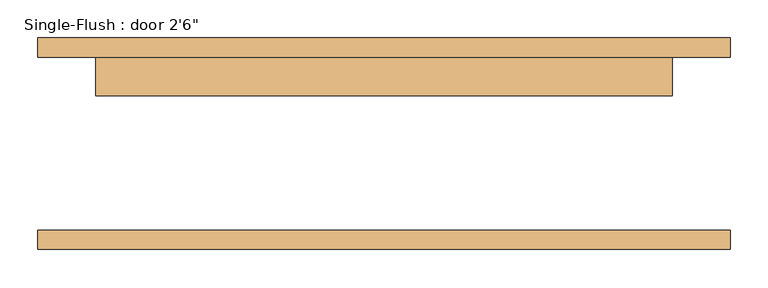
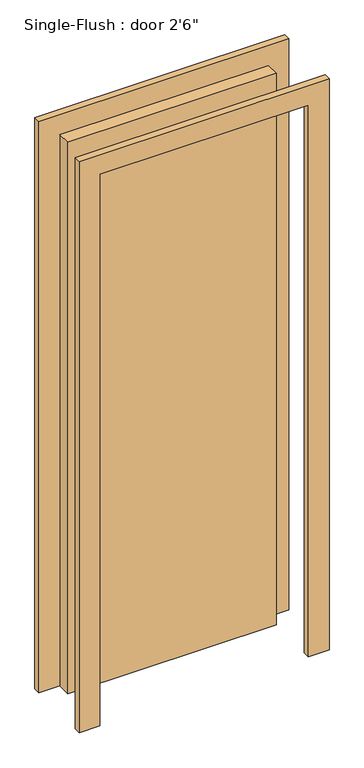
"""IFC4 building model written with IfcOpenShell, lengths in millimetres: door geometry."""

from ifc_helpers import new_model, si_unit, frame, origin, origin_with_axes, place, context, project, spatial, polyline, outline, extrude, source, transform, mapped, element, save


def door_bb98abfd(model_context):
    return source(origin(), model_context, "Body", "SweptSolid", [
        extrude(outline(polyline([(2209.8, -457.2), (0.0, -457.2), (0.0, -381.0), (2133.6, -381.0), (2133.6, 381.0), (0.0, 381.0), (0.0, 457.2), (2209.8, 457.2), (2209.8, -457.2)])), frame((0.0, 114.3, 0.0), z_axis=(0.0, 1.0, 0.0), x_axis=(0.0, 0.0, 1.0)), (0.0, 0.0, 1.0), 25.4),
        extrude(outline(polyline([(2209.8, 457.2), (2209.8, -457.2), (0.0, -457.2), (0.0, -381.0), (2133.6, -381.0), (2133.6, 381.0), (0.0, 381.0), (0.0, 457.2), (2209.8, 457.2)])), frame((0.0, -139.7, 0.0), z_axis=(0.0, 1.0, 0.0), x_axis=(0.0, 0.0, 1.0)), (0.0, 0.0, 1.0), 25.4),
        extrude(outline(polyline([(381.0, 63.5), (-381.0, 63.5), (-381.0, 114.3), (381.0, 114.3), (381.0, 63.5)])), origin_with_axes(), (0.0, 0.0, 1.0), 2133.6),
    ])


if __name__ == "__main__":
    model = new_model("IFC4")
    model_context = context("Model", 3, world=origin())
    ifc_project = project(units=[si_unit("LENGTHUNIT", "METRE", prefix="MILLI")], contexts=[model_context])
    site = spatial("IfcSite", under=ifc_project)
    building = spatial("IfcBuilding", under=site)
    placement = place(None, origin())
    door_shape = door_bb98abfd(model_context)
    element("IfcDoor", 1, ObjectType="Single-Flush : door 2'6\"", at=placement, inside=building, context=model_context, shape_type="MappedRepresentation", body=[
        mapped(door_shape, transform((0.0, 0.0, 0.0), x_axis=(1.0, 0.0, 0.0), y_axis=(0.0, 1.0, 0.0), z_axis=(0.0, 0.0, 1.0))),
    ])
    save(model, "model.ifc")

# Revit data of these elements
# Type "Single-Flush : door 2'6\""
#   Type Mark = "10"
#   Construction Type Id = "MDOOR"
#   Assembly Code = "C1020"
#   Analytic Construction = "Metal"
#   Thickness = 0' - 2"
#   Heat Transfer Coefficient (U) = 0.651978 BTU/(h·ft²·°F)
#   Height = 7' - 0"
#   Trim Projection Ext = 0' - 1"
#   Trim Projection Int = 0' - 1"
#   Trim Width = 0' - 3"
#   Width = 2' - 6"
#   Define Thermal Properties by = 1
#   Door Material = Door - Panel
#   Frame Material = Door - Frame
#   Visual Light Transmittance = 0
#   Solar Heat Gain Coefficient = 0
#   Function = (empty or 0)
#   Wall Closure = (empty or 0)
# Element 1 (IfcDoor, "Single-Flush : door 2'6\"")
#   Materials on its faces: "Door - Frame", "Door - Panel"
# Materials
#   "Door - Panel": class "Wood", colour RGB 210 159 95, transparency 0, Cost = 0
#   "Door - Frame": colour RGB 118 70 51, transparency 0, Cost = 0
